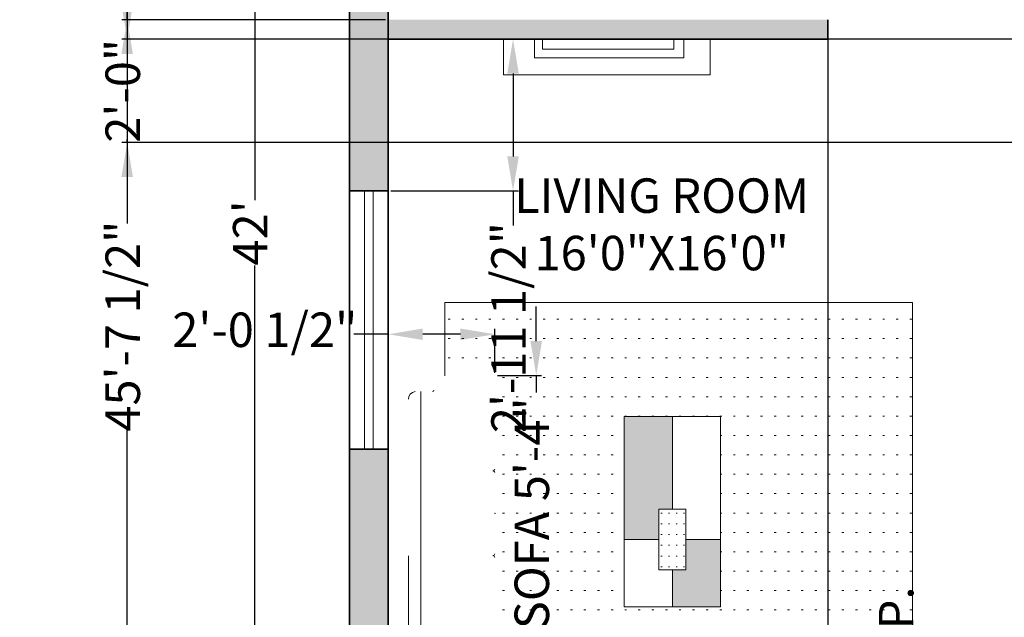
# Model space of a CAD drawing. Units: inches. Extents: x 2408 to 5087, y 2429 to 5085.
# Tile 6 of 12: x 2408 to 2636, y 2676 to 2815. Entities that reach past the tile are written whole.
import ezdxf

# ---------------------------------------------------------------- set-up
doc = ezdxf.new("R2010")
doc.units = ezdxf.units.IN
for name, color, linetype, lineweight in [('A-ANNO-DIMS', 2, 'Continuous', 18), ('A-AREA-IDEN', 6, 'Continuous', 18), ('A-EQPM', 53, 'Continuous', 18), ('A-FLOR-CASE', 8, 'Continuous', 18), ('A-FLOR-PATT', 8, 'Continuous', 13), ('A-FURN', 72, 'Continuous', 18), ('A-FURN-PATT', 251, 'Continuous', 13), ('A-GLAZ', 4, 'Continuous', 18), ('A-WALL', 7, 'Continuous', 35), ('A-WALL-PATT', 252, 'Continuous', 13)]:
    doc.layers.add(name, color=color, linetype=linetype, lineweight=lineweight)
doc.styles.get("Standard").update_dxf_attribs({"font": 'arial.ttf'})
doc.dimstyles.new('ISO-25', dxfattribs={"dimtxt": 8, "dimasz": 8, "dimexe": 1.25, "dimexo": 0.625, "dimtad": 0, "dimdec": 1, "dimlunit": 4, "dimtxsty": 'Standard', "dimcen": 2.5, "dimadec": 0, "dimazin": 0, "dimtfac": 1, "dimtdec": 1, "dimtmove": 0, "dimatfit": 3, "dimfxl": 1, "dimarcsym": 0})

# ---------------------------------------------------------------- blocks, each defined once
blk = doc.blocks.new('*D2')
at = {"layer": 'A-ANNO-DIMS', "color": 0, "lineweight": -2, "transparency": 16777216}
for p, q in [((2483.87, 3017.05), (2461.26, 3017.05)), ((2462.51, 3009.05), (2462.51, 2772.63)), ((2462.51, 2521.05), (2462.51, 2757.48)), ((2483.87, 2513.05), (2461.26, 2513.05))]:
    blk.add_line(p, q, dxfattribs=at)
at = {"layer": 'A-ANNO-DIMS', "color": 0, "transparency": 16777216}
for points in [[(2461.17, 3009.05), (2463.84, 3009.05), (2462.51, 3017.05)], [(2461.17, 2521.05), (2463.84, 2521.05), (2462.51, 2513.05)]]:
    blk.add_solid(points, dxfattribs=at)
at = {"layer": 'Defpoints', "color": 0, "transparency": 16777216}
for p in [(2484.49, 3017.05), (2462.51, 2513.05), (2484.49, 2513.05)]:
    blk.add_point(p, dxfattribs=at)
at = {"layer": 'A-ANNO-DIMS', "color": 0, "transparency": 16777216, "insert": (2462.51, 2765.05), "char_height": 8, "attachment_point": 5, "rotation": 90}
blk.add_mtext("42'", dxfattribs=at)
blk = doc.blocks.new('Clinicians and patient chairs 9_dwgmodels.com')
at = {"color": 0}
for points in [[(-907.9, 0, 0, 0, 0), (-959.6, -11.1, 4.62, 4.62, 0)], [(907.9, 0, 0, 0, 0), (-907.9, 0, 4.62, 4.62, 0)], [(959.6, -11.1, 0, 0, 0), (907.9, 0, 4.62, 4.62, 0)], [(-1015.6, -68.3, 0, 0, 0), (-1025.5, -106.3, 4.62, 4.62, 0)], [(-994.7, -35.9, 0, 0, 0), (-1015.6, -68.3, 4.62, 4.62, 0)], [(-959.6, -11.1, 0, 0, 0), (-994.7, -35.9, 4.62, 4.62, 0)], [(994.7, -35.9, 0, 0, 0), (959.6, -11.1, 4.62, 4.62, 0)], [(1015.6, -68.3, 0, 0, 0), (994.7, -35.9, 4.62, 4.62, 0)], [(1025.5, -106.3, 0, 0, 0), (1015.6, -68.3, 4.62, 4.62, 0)], [(-1025.5, -106.3, 0, 0, 0), (-1025.5, -779.5, 4.62, 4.62, 0)], [(-309.5, -148.3, 0, 0, 0), (-314.5, -150.4, 4.62, 4.62, 0)], [(-308, -148.3, 0, 0, 0), (-309.5, -148.3, 4.62, 4.62, 0)], [(-307.5, -148.3, 0, 0, 0), (-308, -148.3, 4.62, 4.62, 0)], [(242.9, -148.3, 0, 0, 0), (-307.5, -148.3, 4.62, 4.62, 0)], [(242.9, -148.3, 0, 0, 0), (296, -148.3, 4.62, 4.62, 0)], [(296, -148.3, 0, 0, 0), (307.5, -148.3, 4.62, 4.62, 0)], [(308, -148.3, 0, 0, 0), (307.5, -148.3, 4.62, 4.62, 0)], [(309.5, -148.3, 0, 0, 0), (308, -148.3, 4.62, 4.62, 0)], [(309.5, -148.3, 0, 0, 0), (314.5, -150.4, 4.62, 4.62, 0)], [(1025.5, -779.5, 0, 0, 0), (1025.5, -106.3, 4.62, 4.62, 0)], [(1025.5, -779.5, 0, 0, 0), (1025.5, -117.3, 4.62, 4.62, 0)], [(-906.6, -285, 0, 0, 0), (-906.4, -198.1, 4.62, 4.62, 0)], [(-313.4, -149.9, 0, 0, 0), (-318.1, -149.9, 4.62, 4.62, 0)], [(-314.5, -150.4, 0, 0, 0), (-315.7, -159.3, 4.62, 4.62, 0)], [(-315.7, -159.3, 0, 0, 0), (-315.7, -777.3, 4.62, 4.62, 0)], [(849.5, -149.9, 0, 0, 0), (313.4, -149.9, 4.62, 4.62, 0)], [(314.5, -150.4, 0, 0, 0), (315.7, -159.3, 4.62, 4.62, 0)], [(315.7, -159.3, 0, 0, 0), (315.7, -777.3, 4.62, 4.62, 0)], [(315.7, -161.8, 0, 0, 0), (315.7, -777.3, 4.62, 4.62, 0)], [(906.9, -327, 0, 0, 0), (906.4, -199.7, 4.62, 4.62, 0)], [(-906.6, -285, 0, 0, 0), (-906.8, -305.4, 4.62, 4.62, 0)], [(-1023, -329.7, 0, 0, 0), (-1019.2, -332.9, 4.62, 4.62, 0)], [(-1019.8, -340.2, 0, 0, 0), (-1023, -348.6, 4.62, 4.62, 0)], [(-1010.3, -335.9, 0, 0, 0), (-1019.8, -340.2, 4.62, 4.62, 0)], [(-1019.2, -332.9, 0, 0, 0), (-1019, -333, 4.62, 4.62, 0)], [(-1019, -333, 0, 0, 0), (-1018.9, -333.1, 4.62, 4.62, 0)], [(-1013.9, -334.2, 0, 0, 0), (-1018.9, -333.1, 4.62, 4.62, 0)], [(-1013.9, -334.2, 0, 0, 0), (-964.4, -335.7, 4.62, 4.62, 0)], [(-917.1, -337, 0, 0, 0), (-1010.3, -335.9, 4.62, 4.62, 0)], [(-964.4, -335.7, 0, 0, 0), (-927.1, -336.8, 4.62, 4.62, 0)], [(-906.8, -305.4, 0, 0, 0), (-906.9, -324.5, 4.62, 4.62, 0)], [(-906.9, -324.5, 0, 0, 0), (-906.9, -329.8, 4.62, 4.62, 0)], [(906.9, -327, 0, 0, 0), (906.9, -329.9, 4.62, 4.62, 0)], [(964.4, -335.7, 0, 0, 0), (914.9, -337.2, 4.62, 4.62, 0)], [(917.1, -339.4, 0, 0, 0), (1010.3, -338.4, 4.62, 4.62, 0)], [(1013.9, -334.2, 0, 0, 0), (964.4, -335.7, 4.62, 4.62, 0)], [(1010.3, -338.4, 0, 0, 0), (1019.8, -342.7, 4.62, 4.62, 0)], [(1013.9, -334.2, 0, 0, 0), (1018.9, -333.1, 4.62, 4.62, 0)], [(1018.9, -333.1, 0, 0, 0), (1019, -333, 4.62, 4.62, 0)], [(1019.2, -332.9, 0, 0, 0), (1019, -333, 4.62, 4.62, 0)], [(1023, -329.7, 0, 0, 0), (1019.2, -332.9, 4.62, 4.62, 0)], [(1019.8, -342.7, 0, 0, 0), (1023, -351.1, 4.62, 4.62, 0)], [(1023, -351.1, 0, 0, 0), (1022.6, -779.8, 4.62, 4.62, 0)], [(-1025.5, -779.5, 0, 0, 0), (-1022.2, -788.7, 4.62, 4.62, 0)], [(-1022.2, -788.7, 0, 0, 0), (-1021.6, -789.8, 4.62, 4.62, 0)], [(-1021.6, -789.8, 0, 0, 0), (-1020.6, -790.5, 4.62, 4.62, 0)], [(-1020.6, -790.5, 0, 0, 0), (-1013.6, -793.7, 4.62, 4.62, 0)], [(-1013.6, -793.7, 0, 0, 0), (1013.6, -793.7, 4.62, 4.62, 0)], [(1019.8, -788.8, 0, 0, 0), (1013.1, -793.7, 4.62, 4.62, 0)], [(1013.6, -793.7, 0, 0, 0), (1020.6, -790.5, 4.62, 4.62, 0)], [(1022.6, -779.8, 0, 0, 0), (1019.8, -788.8, 4.62, 4.62, 0)], [(1020.6, -790.5, 0, 0, 0), (1021.6, -789.8, 4.62, 4.62, 0)], [(1022.2, -788.7, 0, 0, 0), (1021.6, -789.8, 4.62, 4.62, 0)], [(1022.2, -788.7, 0, 0, 0), (1025.5, -779.5, 4.62, 4.62, 0)]]:
    blk.add_lwpolyline(points, format="xyseb", dxfattribs=at)
for points in [[(-849.5, -149.9), (-318.1, -149.9)], [(-906.5, -241.5), (906.5, -242.3)]]:
    blk.add_lwpolyline(points, dxfattribs=at)
for centre, radius, start, end in [((-851.7, -204.8), 54.9, 87.66794, 174.72556), ((851.7, -204.8), 54.9, 5.27444, 92.33206), ((-916.6, -326.8), 10.2, 267.54544, 342.40568), ((916.9, -329.4), 10, 182.60942, 270.79497), ((-337, -773.8), 21.5, 292.11503, 350.63044), ((-294.5, -773.8), 21.5, 189.36956, 247.88497), ((294.5, -773.8), 21.5, 292.11503, 350.63044), ((336.9, -773.8), 21.5, 189.36956, 247.88497)]:
    blk.add_arc(centre, radius, start, end, dxfattribs=at)
blk.add_point((0, -793.7), dxfattribs=at)
blk = doc.blocks.new('WIN-60x9')
for p, q in [((3.5, 60), (3.5, 0)), ((5.5, 60), (5.5, 0))]:
    blk.add_line(p, q)
blk.add_lwpolyline([(0, 60), (9, 60), (9, 0), (0, 0)], close=True)
blk = doc.blocks.new('TV-FLAT-PANEL')
for points in [[(0, 34.68), (4.32, 34.68), (4.32, 0), (0, 0)], [(0, 32.31), (2.36, 32.31), (2.36, 1.87), (0, 1.87)]]:
    blk.add_lwpolyline(points, close=True)
blk = doc.blocks.new('*D27')
at = {"layer": 'A-ANNO-DIMS', "color": 0, "lineweight": -2, "transparency": 16777216}
for p, q in [((2612.36, 2568.68), (2612.36, 2576.68)), ((2608.98, 2568.68), (2613.61, 2568.68)), ((2612.36, 2550.04), (2612.36, 2560.68)), ((2608.98, 2542.04), (2613.61, 2542.04))]:
    blk.add_line(p, q, dxfattribs=at)
at = {"layer": 'A-ANNO-DIMS', "color": 0, "transparency": 16777216}
for points in [[(2611.02, 2560.68), (2613.69, 2560.68), (2612.36, 2568.68)], [(2611.02, 2550.04), (2613.69, 2550.04), (2612.36, 2542.04)]]:
    blk.add_solid(points, dxfattribs=at)
at = {"layer": 'Defpoints', "color": 0, "transparency": 16777216}
for p in [(2608.36, 2568.68), (2612.36, 2568.68), (2608.36, 2542.04)]:
    blk.add_point(p, dxfattribs=at)
at = {"layer": 'A-ANNO-DIMS', "color": 0, "transparency": 16777216, "insert": (2612.36, 2631.3), "char_height": 8, "attachment_point": 5, "rotation": 90}
blk.add_mtext('PAVER 2\'-2 1/2" TYP.', dxfattribs=at)
blk = doc.blocks.new('*D45')
at = {"layer": 'A-ANNO-DIMS', "color": 0, "lineweight": -2, "transparency": 16777216}
for p, q in [((2525.6, 2657.87), (2525.6, 2661.99)), ((2548.93, 2657.87), (2548.93, 2661.99)), ((2525.6, 2660.74), (2517.6, 2660.74)), ((2540.93, 2660.74), (2533.6, 2660.74))]:
    blk.add_line(p, q, dxfattribs=at)
at = {"layer": 'A-ANNO-DIMS', "color": 0, "transparency": 16777216}
for points in [[(2533.6, 2662.08), (2533.6, 2659.41), (2525.6, 2660.74)], [(2540.93, 2662.08), (2540.93, 2659.41), (2548.93, 2660.74)]]:
    blk.add_solid(points, dxfattribs=at)
at = {"layer": 'Defpoints', "color": 0, "transparency": 16777216}
for p in [(2525.6, 2660.74), (2525.6, 2657.24), (2548.93, 2657.24)]:
    blk.add_point(p, dxfattribs=at)
at = {"layer": 'A-ANNO-DIMS', "color": 0, "transparency": 16777216, "insert": (2461.28, 2660.74), "char_height": 8, "attachment_point": 5}
blk.add_mtext('CHAIR 1\'-11 1/2" TYP.', dxfattribs=at)
blk = doc.blocks.new('*D53')
at = {"layer": 'A-ANNO-DIMS', "color": 0, "lineweight": -2, "transparency": 16777216}
for p, q in [((2527.83, 2739.92), (2527.83, 2747.92)), ((2518.86, 2731.92), (2529.08, 2731.92)), ((2527.83, 2731.92), (2527.83, 2727.96)), ((2527.83, 2667.99), (2527.83, 2671.95)), ((2518.86, 2667.99), (2529.08, 2667.99)), ((2527.83, 2659.99), (2527.83, 2651.99))]:
    blk.add_line(p, q, dxfattribs=at)
at = {"layer": 'A-ANNO-DIMS', "color": 0, "transparency": 16777216}
for points in [[(2526.49, 2739.92), (2529.16, 2739.92), (2527.83, 2731.92)], [(2526.49, 2659.99), (2529.16, 2659.99), (2527.83, 2667.99)]]:
    blk.add_solid(points, dxfattribs=at)
at = {"layer": 'Defpoints', "color": 0, "transparency": 16777216}
for p in [(2518.24, 2731.92), (2527.83, 2731.92), (2518.24, 2667.99)]:
    blk.add_point(p, dxfattribs=at)
at = {"layer": 'A-ANNO-DIMS', "color": 0, "transparency": 16777216, "insert": (2527.83, 2699.95), "char_height": 8, "attachment_point": 5, "rotation": 90}
blk.add_mtext('SOFA 5\'-4"', dxfattribs=at)
blk = doc.blocks.new('*D54')
at = {"layer": 'A-ANNO-DIMS', "color": 0, "lineweight": -2, "transparency": 16777216}
for p, q in [((2493.49, 2741.51), (2485.49, 2741.51)), ((2493.49, 2732.55), (2493.49, 2742.76)), ((2510.24, 2741.51), (2501.49, 2741.51)), ((2518.24, 2732.55), (2518.24, 2742.76))]:
    blk.add_line(p, q, dxfattribs=at)
at = {"layer": 'A-ANNO-DIMS', "color": 0, "transparency": 16777216}
for points in [[(2501.49, 2742.84), (2501.49, 2740.18), (2493.49, 2741.51)], [(2510.24, 2742.84), (2510.24, 2740.18), (2518.24, 2741.51)]]:
    blk.add_solid(points, dxfattribs=at)
at = {"layer": 'Defpoints', "color": 0, "transparency": 16777216}
for p in [(2493.49, 2741.51), (2493.49, 2731.92), (2518.24, 2731.92)]:
    blk.add_point(p, dxfattribs=at)
at = {"layer": 'A-ANNO-DIMS', "color": 0, "transparency": 16777216, "insert": (2464.85, 2741.51), "char_height": 8, "attachment_point": 5}
blk.add_mtext('2\'-0 1/2"', dxfattribs=at)
blk = doc.blocks.new('*D61')
at = {"layer": 'A-ANNO-DIMS', "color": 0, "lineweight": -2, "transparency": 16777216}
for p, q in [((2493.49, 2813.93), (2493.49, 2439.55)), ((2595.49, 2813.93), (2595.49, 2439.55)), ((2501.49, 2440.8), (2533.23, 2440.8)), ((2587.49, 2440.8), (2555.76, 2440.8))]:
    blk.add_line(p, q, dxfattribs=at)
at = {"layer": 'A-ANNO-DIMS', "color": 0, "transparency": 16777216}
for points in [[(2501.49, 2442.13), (2501.49, 2439.47), (2493.49, 2440.8)], [(2587.49, 2442.13), (2587.49, 2439.47), (2595.49, 2440.8)]]:
    blk.add_solid(points, dxfattribs=at)
at = {"layer": 'Defpoints', "color": 0, "transparency": 16777216}
for p in [(2493.49, 2814.55), (2595.49, 2814.55), (2595.49, 2440.8)]:
    blk.add_point(p, dxfattribs=at)
at = {"layer": 'A-ANNO-DIMS', "color": 0, "transparency": 16777216, "insert": (2544.49, 2440.8), "char_height": 8, "attachment_point": 5}
blk.add_mtext('8\'-6"', dxfattribs=at)
blk = doc.blocks.new('*D62')
at = {"layer": 'A-ANNO-DIMS', "color": 0, "lineweight": -2, "transparency": 16777216}
for p, q in [((2432.93, 2875.05), (2432.93, 2883.05)), ((2492.87, 2867.05), (2431.68, 2867.05)), ((2432.93, 2867.05), (2432.93, 2861.54)), ((2432.93, 2814.55), (2432.93, 2820.06)), ((2492.87, 2814.55), (2431.68, 2814.55)), ((2432.93, 2806.55), (2432.93, 2798.55))]:
    blk.add_line(p, q, dxfattribs=at)
at = {"layer": 'A-ANNO-DIMS', "color": 0, "transparency": 16777216}
for points in [[(2431.59, 2875.05), (2434.26, 2875.05), (2432.93, 2867.05)], [(2431.59, 2806.55), (2434.26, 2806.55), (2432.93, 2814.55)]]:
    blk.add_solid(points, dxfattribs=at)
at = {"layer": 'Defpoints', "color": 0, "transparency": 16777216}
for p in [(2432.93, 2867.05), (2493.49, 2867.05), (2493.49, 2814.55)]:
    blk.add_point(p, dxfattribs=at)
at = {"layer": 'A-ANNO-DIMS', "color": 0, "transparency": 16777216, "insert": (2432.93, 2840.8), "char_height": 8, "attachment_point": 5, "rotation": 90}
blk.add_mtext('4\'-4 1/2"', dxfattribs=at)
blk = doc.blocks.new('*D66')
at = {"layer": 'A-ANNO-DIMS', "color": 0, "lineweight": -2, "transparency": 16777216}
for p, q in [((2483.87, 3017.05), (2431.68, 3017.05)), ((2432.93, 3009.05), (2432.93, 2767.25)), ((2432.93, 2477.75), (2432.93, 2719.56)), ((2461.25, 2469.75), (2431.68, 2469.75))]:
    blk.add_line(p, q, dxfattribs=at)
at = {"layer": 'A-ANNO-DIMS', "color": 0, "transparency": 16777216}
for points in [[(2431.59, 3009.05), (2434.26, 3009.05), (2432.93, 3017.05)], [(2431.59, 2477.75), (2434.26, 2477.75), (2432.93, 2469.75)]]:
    blk.add_solid(points, dxfattribs=at)
at = {"layer": 'Defpoints', "color": 0, "transparency": 16777216}
for p in [(2432.93, 3017.05), (2484.49, 3017.05), (2461.88, 2469.75)]:
    blk.add_point(p, dxfattribs=at)
at = {"layer": 'A-ANNO-DIMS', "color": 0, "transparency": 16777216, "insert": (2432.93, 2743.4), "char_height": 8, "attachment_point": 5, "rotation": 90}
blk.add_mtext('45\'-7 1/2"', dxfattribs=at)
blk = doc.blocks.new('*D73')
at = {"layer": 'A-ANNO-DIMS', "color": 0, "lineweight": -2, "transparency": 16777216}
for p, q in [((2494.12, 2810.05), (2523.69, 2810.05)), ((2522.44, 2802.05), (2522.44, 2782.8)), ((2494.12, 2774.8), (2523.69, 2774.8)), ((2522.44, 2774.8), (2522.44, 2766.8))]:
    blk.add_line(p, q, dxfattribs=at)
at = {"layer": 'A-ANNO-DIMS', "color": 0, "transparency": 16777216}
for points in [[(2521.11, 2802.05), (2523.78, 2802.05), (2522.44, 2810.05)], [(2521.11, 2782.8), (2523.78, 2782.8), (2522.44, 2774.8)]]:
    blk.add_solid(points, dxfattribs=at)
at = {"layer": 'Defpoints', "color": 0, "transparency": 16777216}
for p in [(2493.49, 2810.05), (2493.49, 2774.8), (2522.44, 2774.8)]:
    blk.add_point(p, dxfattribs=at)
at = {"layer": 'A-ANNO-DIMS', "color": 0, "transparency": 16777216, "insert": (2522.44, 2743.05), "char_height": 8, "attachment_point": 5, "rotation": 90}
blk.add_mtext('2\'-11 1/2"', dxfattribs=at)
blk = doc.blocks.new('*D79')
at = {"layer": 'A-ANNO-DIMS', "color": 0, "lineweight": -2, "transparency": 16777216}
for p, q in [((2432.93, 2818.05), (2432.93, 2826.05)), ((2693.87, 2810.05), (2431.68, 2810.05)), ((2432.93, 2810.05), (2432.93, 2809.38)), ((2693.87, 2786.05), (2431.68, 2786.05)), ((2432.93, 2786.05), (2432.93, 2786.73)), ((2432.93, 2778.05), (2432.93, 2770.05))]:
    blk.add_line(p, q, dxfattribs=at)
at = {"layer": 'A-ANNO-DIMS', "color": 0, "transparency": 16777216}
for points in [[(2431.59, 2818.05), (2434.26, 2818.05), (2432.93, 2810.05)], [(2431.59, 2778.05), (2434.26, 2778.05), (2432.93, 2786.05)]]:
    blk.add_solid(points, dxfattribs=at)
at = {"layer": 'Defpoints', "color": 0, "transparency": 16777216}
for p in [(2432.93, 2810.05), (2694.49, 2810.05), (2694.49, 2786.05)]:
    blk.add_point(p, dxfattribs=at)
at = {"layer": 'A-ANNO-DIMS', "color": 0, "transparency": 16777216, "insert": (2432.93, 2798.05), "char_height": 8, "attachment_point": 5, "rotation": 90}
blk.add_mtext('2\'-0"', dxfattribs=at)

msp = doc.modelspace()

# ---------------------------------------------------------------- hatches: boundary and pattern name
at = {"layer": 'A-FLOR-PATT'}
h = msp.add_hatch(dxfattribs=at)
h.set_pattern_fill('ACAD_ISO07W100', color=256, scale=0.9)
h.paths.add_polyline_path([(2562.5, 2700.89), (2556.3, 2700.89), (2556.3, 2686.85), (2562.5, 2686.85)], flags=0)
h.paths.add_polyline_path([(2615.08, 2748.91), (2506.63, 2748.91), (2506.63, 2731.92), (2517.79, 2731.92), (2518.12, 2731.8), (2518.26, 2731.5), (2518.24, 2731.53), (2518.24, 2668.18), (2517.9, 2667.99), (2506.63, 2667.99), (2506.63, 2649.35), (2525.6, 2649.35), (2525.6, 2656.74), (2525.67, 2656.76), (2525.66, 2656.79), (2525.7, 2656.79), (2525.74, 2656.78), (2525.93, 2656.85), (2525.94, 2656.85), (2528.05, 2656.85), (2528.14, 2657.1), (2528.15, 2657.1), (2528.16, 2657.12), (2528.24, 2657.12), (2528.43, 2657.16), (2529.11, 2657.19), (2529.97, 2657.24), (2531.76, 2657.24), (2534.59, 2657.13), (2537.27, 2657.14), (2539.94, 2657.13), (2542.78, 2657.24), (2544.57, 2657.24), (2545.42, 2657.19), (2546.38, 2657.15), (2546.5, 2656.79), (2546.66, 2656.85), (2548.6, 2656.85), (2548.82, 2656.85), (2548.84, 2656.79), (2548.87, 2656.79), (2548.87, 2656.71), (2548.96, 2656.45), (2548.93, 2656.53), (2548.93, 2649.35), (2556.54, 2649.35), (2556.54, 2654.76), (2567.14, 2654.76), (2567.14, 2649.35), (2575.28, 2649.35), (2575.28, 2656.74), (2575.34, 2656.76), (2575.34, 2656.79), (2575.38, 2656.79), (2575.42, 2656.78), (2575.61, 2656.85), (2575.61, 2656.85), (2577.73, 2656.85), (2577.82, 2657.1), (2577.83, 2657.1), (2577.84, 2657.12), (2577.92, 2657.12), (2578.11, 2657.16), (2578.79, 2657.19), (2579.64, 2657.24), (2581.43, 2657.24), (2584.27, 2657.13), (2586.94, 2657.14), (2589.62, 2657.13), (2592.46, 2657.24), (2594.25, 2657.24), (2595.1, 2657.19), (2596.05, 2657.15), (2596.18, 2656.79), (2596.34, 2656.85), (2598.28, 2656.85), (2598.5, 2656.85), (2598.52, 2656.79), (2598.55, 2656.79), (2598.55, 2656.71), (2598.64, 2656.45), (2598.61, 2656.53), (2598.61, 2649.35), (2615.08, 2649.35)])
h.paths.add_polyline_path([(2570.6, 2678.23), (2548.2, 2678.23), (2548.2, 2722.4), (2570.6, 2722.4)], flags=16)
h.paths.add_polyline_path([(2562.5, 2686.85), (2556.3, 2686.85), (2556.3, 2700.89), (2562.5, 2700.89)], flags=0)
at = {"layer": 'A-FURN-PATT'}
h = msp.add_hatch(color=256, dxfattribs=at)
h.dxf.hatch_style = 1
h.paths.add_polyline_path([(2559.4, 2722.4), (2548.2, 2722.4), (2548.2, 2693.87), (2556.3, 2693.87), (2556.3, 2700.89), (2559.4, 2700.89)])
h.paths.add_polyline_path([(2570.6, 2693.87), (2562.5, 2693.87), (2562.5, 2686.85), (2559.4, 2686.85), (2559.4, 2678.23), (2570.6, 2678.23)])
h = msp.add_hatch(dxfattribs=at)
h.set_pattern_fill('ACAD_ISO07W100', color=256, scale=0.5)
h.paths.add_polyline_path([(2562.5, 2700.89), (2556.3, 2700.89), (2556.3, 2686.85), (2562.5, 2686.85)])
at = {"layer": 'A-WALL-PATT'}
h = msp.add_hatch(color=256, dxfattribs=at)
h.dxf.hatch_style = 1
h.paths.add_polyline_path([(2493.49, 2613.55), (2523.49, 2613.55), (2523.49, 2622.55), (2493.49, 2622.55), (2493.49, 2714.8), (2484.49, 2714.8), (2484.49, 2497.75), (2493.49, 2497.75)])
h.paths.add_polyline_path([(2613.49, 2615.42), (2613.49, 2622.55), (2583.49, 2622.55), (2583.49, 2613.55), (2613.46, 2613.55, -0.009707)])
h.paths.add_polyline_path([(2823.49, 2634.55), (2814.49, 2634.55), (2814.49, 2622.55), (2694.49, 2622.55), (2694.49, 2670.55), (2706.49, 2670.55), (2706.49, 2675.05), (2694.49, 2675.05), (2694.49, 2750.05), (2685.49, 2750.05), (2685.49, 2622.55), (2661.49, 2622.55), (2661.49, 2613.55), (2814.49, 2613.55), (2814.49, 2522.05), (2688.49, 2522.05), (2688.49, 2513.05), (2823.49, 2513.05)])
h.paths.add_polyline_path([(2823.49, 2837.05), (2814.49, 2837.05), (2814.49, 2819.05), (2685.49, 2819.05), (2685.49, 2786.05), (2694.49, 2786.05), (2694.49, 2810.05), (2814.49, 2810.05), (2814.49, 2772.55), (2823.49, 2772.55)])
h.paths.add_polyline_path([(2694.49, 2964.55), (2595.49, 2964.55), (2595.49, 3008.05), (2601.49, 3008.05), (2601.49, 3017.05), (2484.49, 3017.05), (2484.49, 2972.05), (2493.49, 2972.05), (2493.49, 3008.05), (2586.49, 3008.05), (2586.49, 2955.55), (2685.49, 2955.55), (2685.49, 2854.87), (2694.49, 2854.87)])
h.paths.add_polyline_path([(2493.49, 2867.05), (2595.49, 2867.05), (2595.49, 2876.05), (2493.49, 2876.05), (2493.49, 2912.05), (2484.49, 2912.05), (2484.49, 2774.8), (2493.49, 2774.8)])
h.paths.add_polyline_path([(2595.49, 2814.55), (2493.49, 2814.55), (2493.49, 2810.05), (2595.49, 2810.05)], flags=17)
h.paths.add_polyline_path([(2724.49, 3017.05), (2625.49, 3017.05), (2625.49, 3008.05), (2685.49, 3008.05), (2685.49, 2994.55), (2694.49, 2994.55), (2694.49, 3008.05), (2724.49, 3008.05)])
h.paths.add_polyline_path([(2823.49, 3017.05), (2784.49, 3017.05), (2784.49, 3008.05), (2814.49, 3008.05), (2814.49, 2913.55), (2814.56, 2897.05), (2823.49, 2897.05)])
h.paths.add_polyline_path([(2823.49, 2712.55), (2814.61, 2712.55), (2814.66, 2701.27), (2814.49, 2701.27), (2814.49, 2675.05), (2740.99, 2675.05), (2740.99, 2687.05), (2736.49, 2687.05), (2736.49, 2670.55), (2814.49, 2670.55), (2814.49, 2658.55), (2823.49, 2658.55)], flags=17)

# ---------------------------------------------------------------- linework, layer by layer
at = {"layer": 'A-FLOR-CASE'}
msp.add_lwpolyline([(2520.26, 2810.05), (2568.2, 2810.05), (2568.2, 2801.72), (2520.26, 2801.72)], close=True, dxfattribs=at)
at = {"layer": 'A-FURN'}
for p, q in [((2559.4, 2722.4), (2559.4, 2700.89)), ((2556.3, 2693.87), (2548.2, 2693.87)), ((2562.5, 2693.87), (2570.6, 2693.87)), ((2559.4, 2686.85), (2559.4, 2678.23))]:
    msp.add_line(p, q, dxfattribs=at)
msp.add_lwpolyline([(2598.61, 2649.35), (2615.08, 2649.35), (2615.08, 2748.91), (2506.63, 2748.91), (2506.63, 2731.84)], dxfattribs=at)
for points in [[(2548.2, 2722.4), (2570.6, 2722.4), (2570.6, 2678.23), (2548.2, 2678.23)], [(2556.3, 2700.89), (2562.5, 2700.89), (2562.5, 2686.85), (2556.3, 2686.85)]]:
    msp.add_lwpolyline(points, close=True, dxfattribs=at)
at = {"layer": 'A-WALL'}
for p, q in [((2484.49, 3017.05), (2484.49, 2497.75)), ((2493.49, 2867.05), (2493.49, 2622.55)), ((2595.49, 2814.55), (2595.49, 2810.05)), ((2595.49, 2810.05), (2493.49, 2810.05)), ((2493.49, 2774.8), (2484.49, 2774.8)), ((2493.49, 2714.8), (2484.49, 2714.8))]:
    msp.add_line(p, q, dxfattribs=at)

# ---------------------------------------------------------------- block references
at = {"layer": 'A-EQPM', "rotation": 270.0000000000014}
msp.add_blockref('TV-FLAT-PANEL', (2527.4, 2810.05), dxfattribs=at)
at = {"layer": 'A-FURN', "xscale": 0.0311716531613342, "yscale": 0.0311716531613342, "zscale": 0.0311716531613342, "rotation": 90}
msp.add_blockref('Clinicians and patient chairs 9_dwgmodels.com', (2493.49, 2699.95), dxfattribs=at)
at = {"layer": 'A-GLAZ'}
msp.add_blockref('WIN-60x9', (2484.49, 2714.8), dxfattribs=at)

# ---------------------------------------------------------------- texts
at = {"layer": 'A-AREA-IDEN', "insert": (2505.49, 2777.7), "char_height": 8, "attachment_point": 1}
msp.add_mtext_dynamic_manual_height_columns('\\pxqc;LIVING ROOM\\P16\'0"X16\'0"', width=102.8772, gutter_width=12.5, heights=[0], dxfattribs=at)

# ---------------------------------------------------------------- dimensions: what is measured, and where the dimension line sits
at = {"layer": 'A-ANNO-DIMS'}
for base, p1, p2, angle, override, picture, middle in [((2432.93, 3017.05), (2461.88, 2469.75), (2484.49, 3017.05), 90, {"dimdec": 1, "dimlfac": 1, "dimrnd": 0, "dimzin": 1, "dimdsep": 46, "dimlunit": 4, "dimfrac": 2}, '*D66', (2432.93, 2743.4)), ((2462.51, 2513.05), (2484.49, 3017.05), (2484.49, 2513.05), 90, {"dimclrd": 0, "dimclre": 0, "dimclrt": 0}, '*D2', (2462.51, 2765.05)), ((2432.93, 2867.05), (2493.49, 2814.55), (2493.49, 2867.05), 90, {"dimdec": 1, "dimlfac": 1, "dimrnd": 0, "dimzin": 1, "dimdsep": 46, "dimlunit": 4, "dimfrac": 2}, '*D62', (2432.93, 2840.8)), ((2432.93, 2810.05), (2694.49, 2786.05), (2694.49, 2810.05), 90, {"dimdec": 1, "dimlfac": 1, "dimrnd": 0, "dimzin": 1, "dimdsep": 46, "dimlunit": 4, "dimfrac": 2}, '*D79', (2432.93, 2798.05)), ((2522.443888, 2774.804224), (2493.493888, 2810.054224), (2493.493888, 2774.804224), 270, {"dimdec": 1, "dimlfac": 1, "dimrnd": 0, "dimzin": 1, "dimdsep": 46, "dimlunit": 4, "dimfrac": 2}, '*D73', (2522.443888, 2743.04961963)), ((2493.4939, 2741.5115), (2518.236, 2731.9213), (2493.4939, 2731.9213), 180, {"dimdec": 1, "dimlfac": 1, "dimrnd": 0, "dimzin": 1, "dimdsep": 46, "dimlunit": 4, "dimfrac": 2}, '*D54', (2464.8471, 2741.5115))]:
    dim = msp.add_linear_dim(base=base, p1=p1, p2=p2, angle=angle, dimstyle='ISO-25', override=override, dxfattribs=at)
    dim.commit()
    dim.dimension.update_dxf_attribs({"geometry": picture, "text_midpoint": middle})
dim = msp.add_linear_dim(base=(2595.49, 2440.8), p1=(2493.49, 2814.55), p2=(2595.49, 2814.55), dimstyle='ISO-25', override={"dimdec": 1, "dimlfac": 1, "dimrnd": 0, "dimzin": 1, "dimdsep": 46, "dimlunit": 4, "dimfrac": 2}, dxfattribs=at)
dim.commit()
dim.dimension.update_dxf_attribs({"geometry": '*D61', "text_midpoint": (2544.49, 2440.8)})
for base, p1, p2, angle, text, picture, middle in [((2527.83, 2731.92), (2518.24, 2667.99), (2518.24, 2731.92), 90, 'SOFA <>', '*D53', (2527.83, 2699.95)), ((2525.6, 2660.74), (2548.93, 2657.24), (2525.6, 2657.24), 180, 'CHAIR <> TYP.', '*D45', (2461.28, 2660.74)), ((2612.36, 2568.68), (2608.36, 2542.04), (2608.36, 2568.68), 90, 'PAVER <> TYP.', '*D27', (2612.36, 2631.3))]:
    dim = msp.add_linear_dim(base=base, p1=p1, p2=p2, angle=angle, text=text, dimstyle='ISO-25', override={"dimdec": 1, "dimlfac": 1, "dimrnd": 0, "dimzin": 1, "dimdsep": 46, "dimlunit": 4, "dimfrac": 2}, dxfattribs=at)
    dim.commit()
    dim.dimension.update_dxf_attribs({"geometry": picture, "text_midpoint": middle})

doc.saveas('drawing.dxf')
